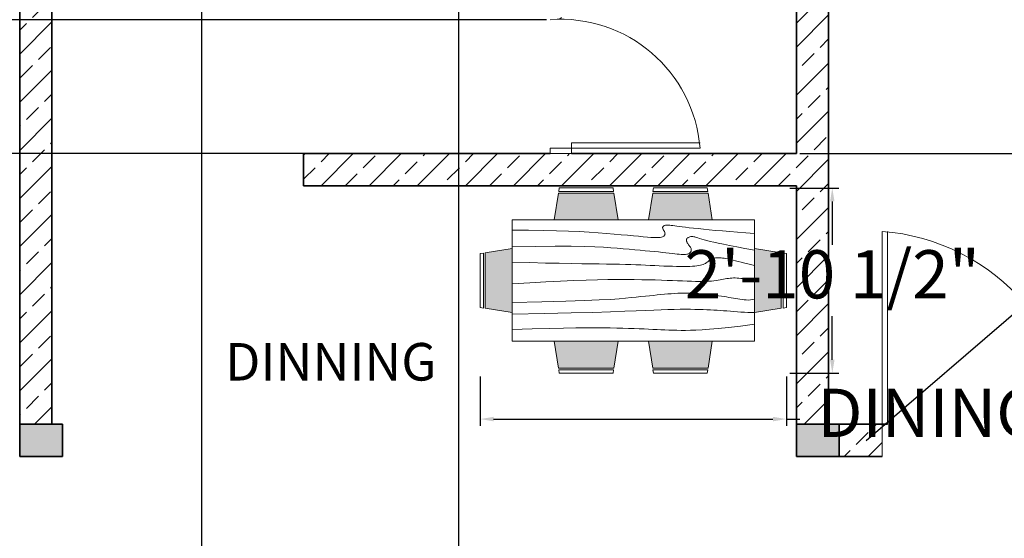
# Model space of a CAD drawing. Units: inches. Extents: x 9689 to 10369, y 10965 to 11626.
# Tile 7 of 11: x 9923 to 10107, y 11359 to 11456. Entities that reach past the tile are written whole.
import ezdxf

# ---------------------------------------------------------------- set-up
doc = ezdxf.new("R2010")
doc.units = ezdxf.units.IN
for name, color, linetype, lineweight in [('A-ANNO-DIMS', 2, 'Continuous', 18), ('A-AREA-IDEN', 7, 'Continuous', 18), ('A-COLS', 7, 'Continuous', 35), ('A-DOOR', 4, 'Continuous', 18), ('A-FURN', 8, 'Continuous', 18), ('A-WALL', 7, 'Continuous', 35), ('A-WALL-PATT', 252, 'Continuous', 13)]:
    doc.layers.add(name, color=color, linetype=linetype, lineweight=lineweight)
doc.layers.add('A-COLS-PATT', color=18, linetype='Continuous', lineweight=13, true_color=0x000000)
doc.layers.add('A-FURN-PATT', color=18, linetype='Continuous', lineweight=13, true_color=0x000000)
doc.styles.get("Standard").update_dxf_attribs({"font": 'arial.ttf'})
doc.dimstyles.new('ISO-25', dxfattribs={"dimtxt": 9, "dimasz": 2.5, "dimexe": 1.25, "dimexo": 0.625, "dimgap": 2, "dimtad": 0, "dimtih": 1, "dimtoh": 1, "dimdec": 1, "dimlunit": 4, "dimtxsty": 'Standard', "dimcen": 2.5, "dimadec": 0, "dimazin": 0, "dimtfac": 0.5, "dimtdec": 1, "dimtmove": 0, "dimatfit": 3, "dimfxl": 1, "dimarcsym": 0})

# ---------------------------------------------------------------- blocks, each defined once
blk = doc.blocks.new('Dining Set - 36 x 72 in.')
for p, q in [((-22, 27.5), (-22.1562, 26.50042)), ((-5.8416, 26.5), (-22.1534, 26.5)), ((-22, 27.5), (-6, 27.5)), ((-5.8437, 26.49966), (-6, 27.5)), ((6, 27.5), (5.8438, 26.50042)), ((22.1584, 26.5), (5.8466, 26.5)), ((6, 27.5), (22, 27.5)), ((22.1563, 26.49966), (22, 27.5)), ((-22.2343, 26.00059), (-23.4847, 17.99762)), ((-22.2304, 26), (-5.7608, 26)), ((-4.5152, 17.99762), (-5.7655, 25.99926)), ((5.7657, 26.00059), (4.5153, 17.99762)), ((5.7696, 26), (22.2392, 26)), ((23.4848, 17.99762), (22.2345, 25.99926)), ((36, 18), (-36, 18)), ((-36, 18), (-36, -18)), ((36, -18), (36, 18)), ((-44.0006, 8.23428), (-35.9976, 9.48474)), ((44.0006, 8.23428), (35.9976, 9.48474)), ((-45.5, 8), (-44.5004, 8.15617)), ((-45.5, 8), (-45.5, -8)), ((-44.5, -8.15843), (-44.5, 8.15338)), ((-44, 8.23041), (-44, -8.23915)), ((44, 8.23041), (44, -8.23915)), ((44.5, -8.15843), (44.5, 8.15338)), ((45.5, 8), (44.5005, 8.15617)), ((45.5, 8), (45.5, -8)), ((-44.4997, -8.15631), (-45.5, -8)), ((-35.9976, -9.48476), (-43.9993, -8.2345)), ((35.9976, -9.48476), (43.9993, -8.2345)), ((44.4997, -8.15631), (45.5, -8)), ((-36, -18), (36, -18)), ((-22.2343, -26.0006), (-23.4847, -17.99762)), ((-4.5152, -17.99762), (-5.7655, -25.99928)), ((5.7657, -26.0006), (4.5153, -17.99762)), ((23.4848, -17.99762), (22.2345, -25.99928)), ((-22.2304, -26), (-5.7608, -26)), ((5.7696, -26), (22.2392, -26)), ((-22, -27.5), (-22.1562, -26.50044)), ((-5.8416, -26.5), (-22.1534, -26.5)), ((-22, -27.5), (-6, -27.5)), ((-5.8437, -26.49967), (-6, -27.5)), ((6, -27.5), (5.8438, -26.50044)), ((22.1584, -26.5), (5.8466, -26.5)), ((6, -27.5), (22, -27.5)), ((22.1563, -26.49967), (22, -27.5))]:
    blk.add_line(p, q)
for points in [[(-36, 15), (-31.1772, 14.97754), (-26.8079, 14.91406), (-22.8538, 14.81543), (-19.276, 14.6875), (-16.0362, 14.53613), (-13.0957, 14.36718), (-10.4159, 14.18652), (-7.9583, 14), (-5.6904, 13.81315), (-3.6035, 13.63021), (-1.6954, 13.45508), (0.0365, 13.29166), (1.5945, 13.14388), (2.9811, 13.01562), (4.1988, 12.9108), (5.25, 12.83333), (6.1393, 12.78613), (6.8802, 12.76823), (7.4883, 12.77767), (7.9792, 12.8125), (8.3685, 12.87077), (8.6719, 12.95052), (8.9049, 13.0498), (9.0833, 13.16666), (9.2205, 13.29899), (9.3216, 13.44401), (9.3895, 13.59879), (9.4271, 13.76041), (9.4373, 13.92594), (9.4232, 14.09245), (9.3875, 14.257), (9.3333, 14.41666), (9.2638, 14.56917), (9.1836, 14.71484), (9.0975, 14.85465), (9.0104, 14.98958), (8.9272, 15.1206), (8.8529, 15.2487), (8.7922, 15.37483), (8.75, 15.5), (8.7305, 15.62467), (8.7344, 15.74739), (8.7617, 15.86621), (8.8125, 15.97916), (8.8867, 16.08431), (8.9844, 16.17968), (9.1055, 16.26334), (9.25, 16.33333), (9.4189, 16.38802), (9.6172, 16.42708), (9.8506, 16.45052), (10.125, 16.45833), (10.4463, 16.45052), (10.8203, 16.42708), (11.2529, 16.38802), (11.75, 16.33333), (12.3184, 16.26318), (12.9694, 16.17838), (13.7151, 16.07991), (14.5677, 15.96875), (15.5395, 15.84586), (16.6426, 15.71224), (17.8893, 15.56884), (19.2917, 15.41666), (20.859, 15.25667), (22.5879, 15.08984), (24.4721, 14.91715), (26.5052, 14.73958), (28.6809, 14.5581), (30.9929, 14.3737), (33.4347, 14.18733), (36, 14)], [(-36, 10), (-28.9766, 10.14274), (-23.1725, 10.20442), (-18.4241, 10.19775), (-14.5677, 10.13541), (-11.4399, 10.03011), (-8.877, 9.89453), (-6.7154, 9.74137), (-4.7917, 9.58333), (-2.9698, 9.43082), (-1.2246, 9.28515), (0.4415, 9.14534), (2.026, 9.01041), (3.5266, 8.87939), (4.9408, 8.7513), (6.266, 8.62516), (7.5, 8.5), (8.6411, 8.37549), (9.6914, 8.2539), (10.6538, 8.13818), (11.5312, 8.03125), (12.3267, 7.93603), (13.043, 7.85547), (13.6831, 7.79248), (14.25, 7.75), (14.7471, 7.7303), (15.1797, 7.73307), (15.5537, 7.75732), (15.875, 7.80208), (16.1494, 7.86637), (16.3828, 7.94922), (16.5811, 8.04964), (16.75, 8.16666), (16.8944, 8.29915), (17.0143, 8.44531), (17.1089, 8.60319), (17.1771, 8.77083), (17.218, 8.94629), (17.2305, 9.1276), (17.2137, 9.31282), (17.1667, 9.5), (17.0895, 9.6875), (16.987, 9.875), (16.8649, 10.0625), (16.7292, 10.25), (16.5856, 10.4375), (16.4401, 10.625), (16.2985, 10.8125), (16.1667, 11), (16.05, 11.18733), (15.9518, 11.3737), (15.8752, 11.5581), (15.8229, 11.73958), (15.798, 11.91715), (15.8034, 12.08984), (15.842, 12.25667), (15.9167, 12.41666), (16.0295, 12.56836), (16.1784, 12.70833), (16.3605, 12.83268), (16.5729, 12.9375), (16.8127, 13.01888), (17.0768, 13.07291), (17.3625, 13.0957), (17.6667, 13.08333), (17.9894, 13.03312), (18.3418, 12.94726), (18.7382, 12.82918), (19.1927, 12.68229), (19.7195, 12.51001), (20.3327, 12.31575), (21.0465, 12.10294), (21.875, 11.875), (22.8357, 11.63354), (23.959, 11.37304), (25.2786, 11.08618), (26.8282, 10.76562), (28.6414, 10.40405), (30.752, 9.99414), (33.1936, 9.52856), (36, 9)], [(-36, 5.5), (-30.7157, 5.3348), (-26.069, 5.20963), (-21.9946, 5.11767), (-18.4271, 5.05208), (-15.3009, 5.00602), (-12.5508, 4.97265), (-10.1112, 4.94515), (-7.9167, 4.91666), (-5.909, 4.88167), (-4.0586, 4.83984), (-2.3429, 4.79215), (-0.7396, 4.73958), (0.7739, 4.6831), (2.22, 4.6237), (3.6213, 4.56233), (5, 4.5), (6.373, 4.43782), (7.7344, 4.3776), (9.0723, 4.32129), (10.375, 4.27083), (11.6309, 4.22819), (12.8281, 4.19531), (13.9551, 4.17415), (15, 4.16666), (15.954, 4.17448), (16.819, 4.19791), (17.6001, 4.23698), (18.3021, 4.29166), (18.9299, 4.36198), (19.4883, 4.44791), (19.9823, 4.54948), (20.4167, 4.66666), (20.7969, 4.79899), (21.1302, 4.94401), (21.4245, 5.09879), (21.6875, 5.26041), (21.9271, 5.42594), (22.1511, 5.59245), (22.3672, 5.757), (22.5834, 5.91666), (22.8065, 6.06868), (23.0404, 6.21093), (23.2879, 6.34147), (23.5521, 6.45833), (23.8358, 6.55957), (24.142, 6.64323), (24.4735, 6.70735), (24.8334, 6.75), (25.2235, 6.76969), (25.642, 6.76692), (26.0858, 6.74267), (26.5521, 6.69791), (27.0379, 6.63362), (27.5404, 6.55078), (28.0565, 6.45036), (28.5834, 6.33333), (29.1242, 6.19987), (29.7071, 6.04687), (30.3661, 5.87044), (31.1354, 5.66666), (32.0493, 5.43164), (33.142, 5.16146), (34.4475, 4.85221), (36, 4.5)], [(-36, -1), (-30.7915, -0.6591), (-26.0195, -0.38216), (-21.6519, -0.16284), (-17.6563, 0.00521), (-14.0005, 0.12833), (-10.6523, 0.21289), (-7.5796, 0.26522), (-4.75, 0.29166), (-2.134, 0.29793), (0.2878, 0.28711), (2.5317, 0.26163), (4.6146, 0.22396), (6.5529, 0.17651), (8.3633, 0.12174), (10.0623, 0.06209), (11.6667, 0), (13.1899, -0.06201), (14.6341, -0.1211), (15.9982, -0.17432), (17.2813, -0.21875), (18.4823, -0.25147), (19.6003, -0.26953), (20.6343, -0.27002), (21.5834, -0.25), (22.4481, -0.20768), (23.2357, -0.14584), (23.9549, -0.06836), (24.6146, 0.02083), (25.2235, 0.11784), (25.7904, 0.21875), (26.3241, 0.31966), (26.8334, 0.41666), (27.3265, 0.50618), (27.8099, 0.58593), (28.2894, 0.65397), (28.7709, 0.70833), (29.2601, 0.74707), (29.763, 0.76823), (30.2855, 0.76985), (30.8334, 0.75), (31.4088, 0.70784), (31.9994, 0.64713), (32.589, 0.57275), (33.1615, 0.48958), (33.7008, 0.4025), (34.1908, 0.3164), (34.6153, 0.23616), (34.9584, 0.16666), (35.2099, 0.11165), (35.3848, 0.07031), (35.504, 0.04069), (35.5886, 0.02083), (35.6594, 0.00879), (35.7377, 0.0026), (35.8442, 0.00032), (36, 0)], [(-36, -6.5), (-27.1843, -6.31267), (-20.084, -6.1263), (-14.469, -5.9419), (-10.1094, -5.76042), (-6.7752, -5.58285), (-4.2363, -5.41016), (-2.2629, -5.24333), (-0.625, -5.08334), (0.8708, -4.93099), (2.2715, -4.78646), (3.5872, -4.64974), (4.8281, -4.52084), (6.0046, -4.39974), (7.127, -4.28646), (8.2053, -4.18099), (9.25, -4.08334), (10.2705, -3.99382), (11.2734, -3.91407), (12.2647, -3.84603), (13.25, -3.79167), (14.2354, -3.75293), (15.2266, -3.73177), (16.2295, -3.73015), (17.25, -3.75), (18.2912, -3.79248), (19.3451, -3.85547), (20.4009, -3.93604), (21.4479, -4.03125), (22.4754, -4.13819), (23.4727, -4.25391), (24.4289, -4.37549), (25.3334, -4.5), (26.1785, -4.62492), (26.9694, -4.74935), (27.7145, -4.87281), (28.4219, -4.99479), (29.1, -5.11483), (29.7572, -5.23242), (30.4016, -5.34709), (31.0417, -5.45834), (31.6837, -5.56437), (32.3262, -5.65821), (32.9658, -5.73153), (33.599, -5.77604), (34.2224, -5.78345), (34.8327, -5.74545), (35.4264, -5.65373), (36, -5.5)], [(-36, -10), (-26.4022, -9.81299), (-18.4675, -9.62891), (-11.9839, -9.45069), (-6.7396, -9.28125), (-2.5226, -9.12354), (0.8789, -8.98047), (3.6769, -8.85498), (6.0833, -8.75), (8.2767, -8.66765), (10.3021, -8.60677), (12.1712, -8.56543), (13.8958, -8.54167), (15.4876, -8.53353), (16.9583, -8.53907), (18.3197, -8.55632), (19.5834, -8.58334), (20.7616, -8.61841), (21.8685, -8.66081), (22.9188, -8.71004), (23.9271, -8.76563), (24.9081, -8.82707), (25.8763, -8.89388), (26.8465, -8.96558), (27.8334, -9.04167), (28.8474, -9.12118), (29.8828, -9.20117), (30.93, -9.27824), (31.9792, -9.34896), (33.0205, -9.40991), (34.0443, -9.45768), (35.0407, -9.48885), (36, -9.5)], [(-36, -14.5), (-30.0881, -14.33513), (-25.0332, -14.21224), (-20.7312, -14.12647), (-17.0781, -14.07292), (-13.97, -14.04671), (-11.3027, -14.04297), (-8.9724, -14.05681), (-6.875, -14.08334), (-4.9224, -14.11833), (-3.0905, -14.16016), (-1.3709, -14.20785), (0.2448, -14.26042), (1.7647, -14.3169), (3.1973, -14.3763), (4.5507, -14.43767), (5.8333, -14.5), (7.0554, -14.5621), (8.235, -14.62175), (9.3922, -14.67652), (10.5469, -14.72396), (11.7192, -14.76164), (12.929, -14.78711), (14.1965, -14.79794), (15.5417, -14.79167), (16.9933, -14.76424), (18.6152, -14.70508), (20.4804, -14.60197), (22.6615, -14.44271), (25.2312, -14.21509), (28.2624, -13.9069), (31.8277, -13.50594), (36, -13)]]:
    blk.add_lwpolyline(points)
blk = doc.blocks.new('DOOR-SWING-24')
for p, q in [((4, 2), (28, 2)), ((4, 2), (4, 0)), ((0, 1), (4, 1)), ((0, 1), (0, 0)), ((0, 0), (4, 0)), ((4, 1), (28, 1))]:
    blk.add_line(p, q)
blk.add_arc((2, -1), 26.08, 4.3987, 94.3987)
blk = doc.blocks.new('DOOR-SWING-36')
for p, q in [((0, 6), (0, 42)), ((1, 6), (1, 42)), ((0, 6), (0, 0))]:
    blk.add_line(p, q)
blk.add_arc((-3, 3), 39.12, 355.6013, 85.6013)
blk = doc.blocks.new('*D52')
at = {"layer": 'A-ANNO-DIMS', "color": 0, "lineweight": -2, "transparency": 16777216}
for p, q in [((10009.02, 11389.55), (10009.02, 11380.35)), ((10066.18, 11389.55), (10066.18, 11380.35)), ((10011.52, 11381.6), (10063.68, 11381.6)), ((10066.18, 11381.6), (10068.68, 11381.6))]:
    blk.add_line(p, q, dxfattribs=at)
at = {"layer": 'A-ANNO-DIMS', "color": 0, "transparency": 16777216}
for points in [[(10011.52, 11382.02), (10011.52, 11381.18), (10009.02, 11381.6)], [(10063.68, 11382.02), (10063.68, 11381.18), (10066.18, 11381.6)]]:
    blk.add_solid(points, dxfattribs=at)
at = {"layer": 'Defpoints', "color": 0, "transparency": 16777216}
for p in [(10009.02, 11390.17), (10066.18, 11390.17), (10066.18, 11381.6)]:
    blk.add_point(p, dxfattribs=at)
at = {"layer": 'A-ANNO-DIMS', "color": 0, "transparency": 16777216, "insert": (10120.14, 11381.6), "char_height": 9, "attachment_point": 5}
blk.add_mtext('DINING SET 4\'-9"', dxfattribs=at)
blk = doc.blocks.new('*D53')
at = {"layer": 'A-ANNO-DIMS', "color": 0, "lineweight": -2, "transparency": 16777216}
for p, q in [((10066.81, 11424.72), (10076, 11424.72)), ((10074.75, 11422.22), (10074.75, 11414.1)), ((10074.75, 11392.67), (10074.75, 11400.79)), ((10066.81, 11390.17), (10076, 11390.17))]:
    blk.add_line(p, q, dxfattribs=at)
at = {"layer": 'A-ANNO-DIMS', "color": 0, "transparency": 16777216}
for points in [[(10074.34, 11422.22), (10075.17, 11422.22), (10074.75, 11424.72)], [(10074.34, 11392.67), (10075.17, 11392.67), (10074.75, 11390.17)]]:
    blk.add_solid(points, dxfattribs=at)
at = {"layer": 'Defpoints', "color": 0, "transparency": 16777216}
for p in [(10066.18, 11424.72), (10074.75, 11424.72), (10066.18, 11390.17)]:
    blk.add_point(p, dxfattribs=at)
at = {"layer": 'A-ANNO-DIMS', "color": 0, "transparency": 16777216, "insert": (10074.75, 11407.45), "char_height": 9, "attachment_point": 5}
blk.add_mtext('2\'-10 1/2"', dxfattribs=at)
blk = doc.blocks.new('*D81')
at = {"layer": 'A-ANNO-DIMS', "color": 0, "lineweight": -2, "transparency": 16777216}
for p, q in [((10068.68, 11529.63), (10287.21, 11529.63)), ((10285.96, 11527.13), (10285.96, 11487.03)), ((10285.96, 11433.63), (10285.96, 11473.73)), ((10068.68, 11431.13), (10287.21, 11431.13))]:
    blk.add_line(p, q, dxfattribs=at)
at = {"layer": 'A-ANNO-DIMS', "color": 0, "transparency": 16777216}
for points in [[(10285.54, 11527.13), (10286.37, 11527.13), (10285.96, 11529.63)], [(10285.54, 11433.63), (10286.37, 11433.63), (10285.96, 11431.13)]]:
    blk.add_solid(points, dxfattribs=at)
at = {"layer": 'Defpoints', "color": 0, "transparency": 16777216}
for p in [(10068.06, 11529.63), (10285.96, 11529.63), (10068.06, 11431.13)]:
    blk.add_point(p, dxfattribs=at)
at = {"layer": 'A-ANNO-DIMS', "color": 0, "transparency": 16777216, "insert": (10285.96, 11480.38), "char_height": 9, "attachment_point": 5}
blk.add_mtext('8\'-2 1/2"', dxfattribs=at)
blk = doc.blocks.new('*D97')
at = {"layer": 'A-ANNO-DIMS', "color": 0, "lineweight": -2, "transparency": 16777216}
for p, q in [((9957.06, 11321.26), (9957.06, 11613.7)), ((10005.06, 11321.26), (10005.06, 11613.7)), ((9959.56, 11612.45), (9966.91, 11612.45)), ((10002.56, 11612.45), (9995.2, 11612.45))]:
    blk.add_line(p, q, dxfattribs=at)
at = {"layer": 'A-ANNO-DIMS', "color": 0, "transparency": 16777216}
for points in [[(9959.56, 11612.87), (9959.56, 11612.04), (9957.06, 11612.45)], [(10002.56, 11612.87), (10002.56, 11612.04), (10005.06, 11612.45)]]:
    blk.add_solid(points, dxfattribs=at)
at = {"layer": 'Defpoints', "color": 0, "transparency": 16777216}
for p in [(10005.06, 11612.45), (9957.06, 11320.63), (10005.06, 11320.63)]:
    blk.add_point(p, dxfattribs=at)
at = {"layer": 'A-ANNO-DIMS', "color": 0, "transparency": 16777216, "insert": (9981.06, 11612.45), "char_height": 9, "attachment_point": 5}
blk.add_mtext('4\'-0"', dxfattribs=at)
blk = doc.blocks.new('*D110')
at = {"layer": 'A-ANNO-DIMS', "color": 0, "lineweight": -2, "transparency": 16777216}
for p, q in [((10021.43, 11456.13), (9758.91, 11456.13)), ((9760.16, 11453.63), (9760.16, 11450.15)), ((9760.16, 11433.63), (9760.16, 11437.11)), ((10021.43, 11431.13), (9758.91, 11431.13))]:
    blk.add_line(p, q, dxfattribs=at)
at = {"layer": 'A-ANNO-DIMS', "color": 0, "transparency": 16777216}
for points in [[(9759.74, 11453.63), (9760.57, 11453.63), (9760.16, 11456.13)], [(9759.74, 11433.63), (9760.57, 11433.63), (9760.16, 11431.13)]]:
    blk.add_solid(points, dxfattribs=at)
at = {"layer": 'Defpoints', "color": 0, "transparency": 16777216}
for p in [(9760.16, 11456.13), (10022.06, 11456.13), (10022.06, 11431.13)]:
    blk.add_point(p, dxfattribs=at)
at = {"layer": 'A-ANNO-DIMS', "color": 0, "transparency": 16777216, "insert": (9760.16, 11443.63), "char_height": 9, "attachment_point": 5}
blk.add_mtext('2\'-1"', dxfattribs=at)
blk = doc.blocks.new('*D119')
at = {"layer": 'A-ANNO-DIMS', "color": 0, "lineweight": -2, "transparency": 16777216}
for p, q in [((10128.57, 11418.36), (10112.65, 11404.71)), ((10131.07, 11418.36), (10128.57, 11418.36)), ((10081.06, 11377.63), (10110.76, 11403.09))]:
    blk.add_line(p, q, dxfattribs=at)
at = {"layer": 'A-ANNO-DIMS', "color": 0, "transparency": 16777216}
blk.add_solid([(10112.38, 11405.03), (10112.92, 11404.4), (10110.76, 11403.09)], dxfattribs=at)
at = {"layer": 'Defpoints', "color": 0, "transparency": 16777216}
for p in [(10110.76, 11403.09), (10081.06, 11377.63)]:
    blk.add_point(p, dxfattribs=at)
at = {"layer": 'A-ANNO-DIMS', "color": 0, "transparency": 16777216, "insert": (10149.34, 11418.36), "char_height": 9, "attachment_point": 5}
blk.add_mtext('R3\'-3"', dxfattribs=at)

msp = doc.modelspace()

# ---------------------------------------------------------------- hatches: boundary and pattern name
at = {"layer": 'A-COLS-PATT'}
h = msp.add_hatch(color=256, dxfattribs=at)
h.dxf.hatch_style = 1
h.paths.add_polyline_path([(9931.06, 11380.63), (9929.06, 11380.63), (9923.06, 11380.63), (9923.06, 11374.63), (9929.06, 11374.63), (9931.06, 11374.63)])
h.paths.add_polyline_path([(10076.06, 11380.63), (10074.06, 11380.63), (10068.06, 11380.63), (10068.06, 11374.63), (10074.06, 11374.63), (10076.06, 11374.63)])
at = {"layer": 'A-FURN-PATT'}
h = msp.add_hatch(color=256, dxfattribs=at)
h.dxf.hatch_style = 1
h.paths.add_polyline_path([(10033.98, 11423.78), (10023.64, 11423.78), (10022.85, 11418.75), (10034.77, 11418.75)])
h.paths.add_polyline_path([(10051.57, 11423.78), (10041.22, 11423.78), (10040.44, 11418.75), (10052.35, 11418.75)])
h.paths.add_polyline_path([(10014.99, 11413.4), (10009.97, 11412.62), (10009.97, 11402.27), (10014.99, 11401.49)])
h.paths.add_polyline_path([(10034.77, 11396.14), (10022.85, 11396.14), (10023.64, 11391.12), (10033.98, 11391.12)])
h.paths.add_polyline_path([(10052.35, 11396.14), (10040.44, 11396.14), (10041.22, 11391.12), (10051.57, 11391.12)])
h.paths.add_polyline_path([(10065.24, 11412.62), (10060.21, 11413.4), (10060.21, 11401.49), (10065.24, 11402.27)])
at = {"layer": 'A-WALL-PATT'}
h = msp.add_hatch(dxfattribs=at)
h.set_pattern_fill('ANSI33', color=256)
h.paths.add_polyline_path([(9843.06, 11538.63), (9811.06, 11538.63), (9811.06, 11529.63), (9843.06, 11529.63)])
h.paths.add_polyline_path([(9923.06, 11538.63), (9891.06, 11538.63), (9891.06, 11529.63), (9923.06, 11529.63)])
h.paths.add_polyline_path([(9929.06, 11527.63), (9923.06, 11527.63), (9923.06, 11380.63), (9929.06, 11380.63)])
h.paths.add_polyline_path([(9939.06, 11538.63), (9929.06, 11538.63), (9929.06, 11529.63), (9939.06, 11529.63, -0.071068)])
h.paths.add_polyline_path([(10035.06, 11538.63), (10013.06, 11538.63), (10013.06, 11529.63), (10022.06, 11529.63), (10022.06, 11507.38), (10022.06, 11502.38), (10022.06, 11482.38), (10022.06, 11478.38), (10022.06, 11456.13, -0.038405), (10026.06, 11456.13), (10026.06, 11502.38), (10026.06, 11529.63), (10035.06, 11529.63)])
h.paths.add_polyline_path([(10068.06, 11538.63), (10059.06, 11538.63), (10059.06, 11529.63), (10068.06, 11529.63)])
h.paths.add_polyline_path([(10074.06, 11527.63), (10068.06, 11527.63), (10068.06, 11431.13), (10026.06, 11431.13), (10022.06, 11431.13), (9980.06, 11431.13), (9976.06, 11431.13), (9976.06, 11425.13), (10068.06, 11425.13), (10068.06, 11380.63), (10074.06, 11380.63)])
h.paths.add_polyline_path([(10124.56, 11538.63), (10074.06, 11538.63), (10074.06, 11529.63), (10124.56, 11529.63)])
h.paths.add_polyline_path([(9980.06, 11507.38), (9980.06, 11529.63), (9989.06, 11529.63), (9989.06, 11538.63), (9976.06, 11538.63), (9976.06, 11529.63), (9976.06, 11503.38), (9976.06, 11483.38), (9976.06, 11478.38), (9980.06, 11478.38), (9997.06, 11478.38, -0.038405), (9997.06, 11482.38), (9980.06, 11482.38)])
h.paths.add_polyline_path([(10235.06, 11538.63), (10184.56, 11538.63), (10184.56, 11529.63), (10235.06, 11529.63)])
h.paths.add_polyline_path([(10244.06, 11527.63), (10235.06, 11527.63), (10235.06, 11485.13), (10244.06, 11485.13)])
h.paths.add_polyline_path([(10244.06, 11425.13), (10235.06, 11425.13), (10235.06, 11380.63), (10244.06, 11380.63)])
h.paths.add_polyline_path([(10233.06, 11380.63), (10120.06, 11380.63, -0.038405), (10120.06, 11374.63), (10133.04, 11374.63), (10133.04, 11326.63), (10120.06, 11326.63, -0.038405), (10120.06, 11320.63), (10149.19, 11320.63), (10149.19, 11326.63), (10136.04, 11326.63), (10136.04, 11374.63), (10233.06, 11374.63)])
h.paths.add_polyline_path([(10084.06, 11380.63), (10076.06, 11380.63), (10076.06, 11374.63), (10084.06, 11374.63)])
h.paths.add_polyline_path([(10244.06, 11374.63), (10235.06, 11374.63), (10235.06, 11362.63), (10244.06, 11362.63)])
h.paths.add_polyline_path([(10244.06, 11338.63), (10235.06, 11338.63), (10235.06, 11326.63), (10244.06, 11326.63)])
h.paths.add_polyline_path([(10233.06, 11326.63), (10173.19, 11326.63, -0.055385), (10173.19, 11320.63), (10233.06, 11320.63)], flags=0)
h.paths.add_polyline_path([(10244.06, 11320.63), (10235.06, 11320.63), (10235.06, 11273.63), (10244.06, 11273.63)])
h = msp.add_hatch(dxfattribs=at)
h.set_pattern_fill('ANSI36', color=256)
h.paths.add_polyline_path([(10233.06, 11326.63), (10173.19, 11326.63, -0.055385), (10173.19, 11320.63), (10233.06, 11320.63)])
h.paths.add_polyline_path([(10244.06, 11213.63), (10235.06, 11213.63), (10235.06, 11166.63), (10244.06, 11166.63)])
h.paths.add_polyline_path([(10233.06, 11166.63), (10184.56, 11166.63), (10184.56, 11157.63), (10233.06, 11157.63)])
h.paths.add_polyline_path([(10124.56, 11166.63), (10074.06, 11166.63), (10074.06, 11157.63), (10124.56, 11157.63)])
h.paths.add_polyline_path([(10074.06, 11318.63), (10068.06, 11318.63), (10068.06, 11168.63), (10074.06, 11168.63)])
h.paths.add_polyline_path([(10068.06, 11166.63), (10011.06, 11166.63), (10011.06, 11157.63), (10068.06, 11157.63)])
h.paths.add_polyline_path([(10011.06, 11318.63), (10005.06, 11318.63), (10005.06, 11168.63), (10011.06, 11168.63)])
h.paths.add_polyline_path([(10005.06, 11166.63), (9985.06, 11166.63), (9985.06, 11157.63), (10005.06, 11157.63)])
h.paths.add_polyline_path([(9937.06, 11166.63), (9898.06, 11166.63), (9898.06, 11157.63), (9937.06, 11157.63, -0.042779)])
h.paths.add_polyline_path([(9850.06, 11166.63), (9813.06, 11166.63), (9813.06, 11157.63), (9850.06, 11157.63)])
h.paths.add_polyline_path([(9811.06, 11213.63), (9802.06, 11213.63), (9802.06, 11166.63), (9811.06, 11166.63)])
h.paths.add_polyline_path([(9811.06, 11320.63), (9802.06, 11320.63), (9802.06, 11273.63), (9811.06, 11273.63)])
h.paths.add_polyline_path([(9811.06, 11439.11), (9802.06, 11439.11), (9802.06, 11326.63), (9811.06, 11326.63)])
h.paths.add_polyline_path([(9957.06, 11326.63), (9813.06, 11326.63), (9813.06, 11320.63), (9957.06, 11320.63)])
h.paths.add_polyline_path([(9811.06, 11527.63), (9802.06, 11527.63), (9802.06, 11499.11), (9811.06, 11499.11)])

# ---------------------------------------------------------------- linework, layer by layer
at = {"layer": 'A-COLS'}
for p, q in [((9929.06, 11380.63), (9923.06, 11380.63)), ((9929.06, 11380.63), (9931.06, 11380.63)), ((9931.06, 11380.63), (9931.06, 11374.63)), ((10074.06, 11380.63), (10068.06, 11380.63)), ((10076.06, 11380.63), (10076.06, 11374.63)), ((9929.06, 11374.63), (9923.06, 11374.63)), ((9929.06, 11374.63), (9931.06, 11374.63)), ((10074.06, 11374.63), (10068.06, 11374.63))]:
    msp.add_line(p, q, dxfattribs=at)
at = {"layer": 'A-WALL'}
for p, q in [((9923.06, 11374.63), (9923.06, 11529.63)), ((9929.06, 11380.63), (9929.06, 11529.63)), ((9929.06, 11431.13), (9929.06, 11529.63)), ((10068.06, 11529.63), (10068.06, 11431.13)), ((10074.06, 11529.63), (10074.06, 11380.63)), ((9976.06, 11431.13), (9976.06, 11425.13)), ((9980.06, 11431.13), (9976.06, 11431.13)), ((10022.06, 11431.13), (9980.06, 11431.13)), ((10068.06, 11431.13), (10026.06, 11431.13)), ((10068.06, 11425.13), (9976.06, 11425.13)), ((10068.06, 11425.13), (10068.06, 11374.63)), ((10074.06, 11380.63), (10085.06, 11380.63)), ((10074.06, 11374.63), (10084.06, 11374.63))]:
    msp.add_line(p, q, dxfattribs=at)

# ---------------------------------------------------------------- block references
at = {"layer": 'A-DOOR'}
for name, p in [('DOOR-SWING-24', (10022.06, 11431.13)), ('DOOR-SWING-36', (10084.06, 11374.63))]:
    msp.add_blockref(name, p, dxfattribs=at)
at = {"layer": 'A-FURN', "xscale": 0.6281026196428844, "yscale": 0.6281026196428844, "zscale": 0.6281026196428844}
msp.add_blockref('Dining Set - 36 x 72 in.', (10037.6, 11407.45), dxfattribs=at)

# ---------------------------------------------------------------- texts
at = {"layer": 'A-AREA-IDEN', "insert": (9961.42, 11395.79), "char_height": 7, "attachment_point": 1}
msp.add_mtext_dynamic_manual_height_columns('{\\fArial|b1|i0|c0|p34;DINNING}', width=73.2317, gutter_width=12.5, heights=[0], dxfattribs=at)

# ---------------------------------------------------------------- dimensions: what is measured, and where the dimension line sits
at = {"layer": 'A-ANNO-DIMS'}
dim = msp.add_linear_dim(base=(10005.06, 11612.45), p1=(9957.06, 11320.63), p2=(10005.06, 11320.63), dimstyle='ISO-25', override={"dimdec": 1, "dimlfac": 1, "dimrnd": 0, "dimzin": 1, "dimdsep": 46, "dimlunit": 4, "dimfrac": 2}, dxfattribs=at)
dim.commit()
dim.dimension.update_dxf_attribs({"geometry": '*D97', "text_midpoint": (9981.06, 11612.45)})
for base, p1, p2, picture, middle in [((10285.96, 11529.63), (10068.06, 11431.13), (10068.06, 11529.63), '*D81', (10285.96, 11480.38)), ((9760.16, 11456.13), (10022.06, 11431.13), (10022.06, 11456.13), '*D110', (9760.16, 11443.63)), ((10074.7542, 11424.7191), (10066.1806, 11390.1734), (10066.1806, 11424.7191), '*D53', (10074.7542, 11407.4462))]:
    dim = msp.add_linear_dim(base=base, p1=p1, p2=p2, angle=90, dimstyle='ISO-25', override={"dimdec": 1, "dimlfac": 1, "dimrnd": 0, "dimzin": 1, "dimdsep": 46, "dimlunit": 4, "dimfrac": 2}, dxfattribs=at)
    dim.commit()
    dim.dimension.update_dxf_attribs({"geometry": picture, "text_midpoint": middle})
dim = msp.add_radius_dim(center=(10081.06, 11377.63), mpoint=(10110.76, 11403.09), dimstyle='ISO-25', override={"dimdec": 1, "dimlfac": 1, "dimrnd": 0, "dimzin": 1, "dimdsep": 46, "dimlunit": 4, "dimfrac": 2}, dxfattribs=at)
dim.commit()
dim.dimension.update_dxf_attribs({"geometry": '*D119', "text_midpoint": (10149.34, 11418.36), "dimtype": 164})
dim = msp.add_linear_dim(base=(10066.18, 11381.6), p1=(10009.02, 11390.17), p2=(10066.18, 11390.17), text='DINING SET <>', dimstyle='ISO-25', override={"dimdec": 1, "dimlfac": 1, "dimrnd": 0, "dimzin": 1, "dimdsep": 46, "dimlunit": 4, "dimfrac": 2}, dxfattribs=at)
dim.commit()
dim.dimension.update_dxf_attribs({"geometry": '*D52', "text_midpoint": (10120.14, 11381.6)})

doc.saveas('drawing.dxf')
